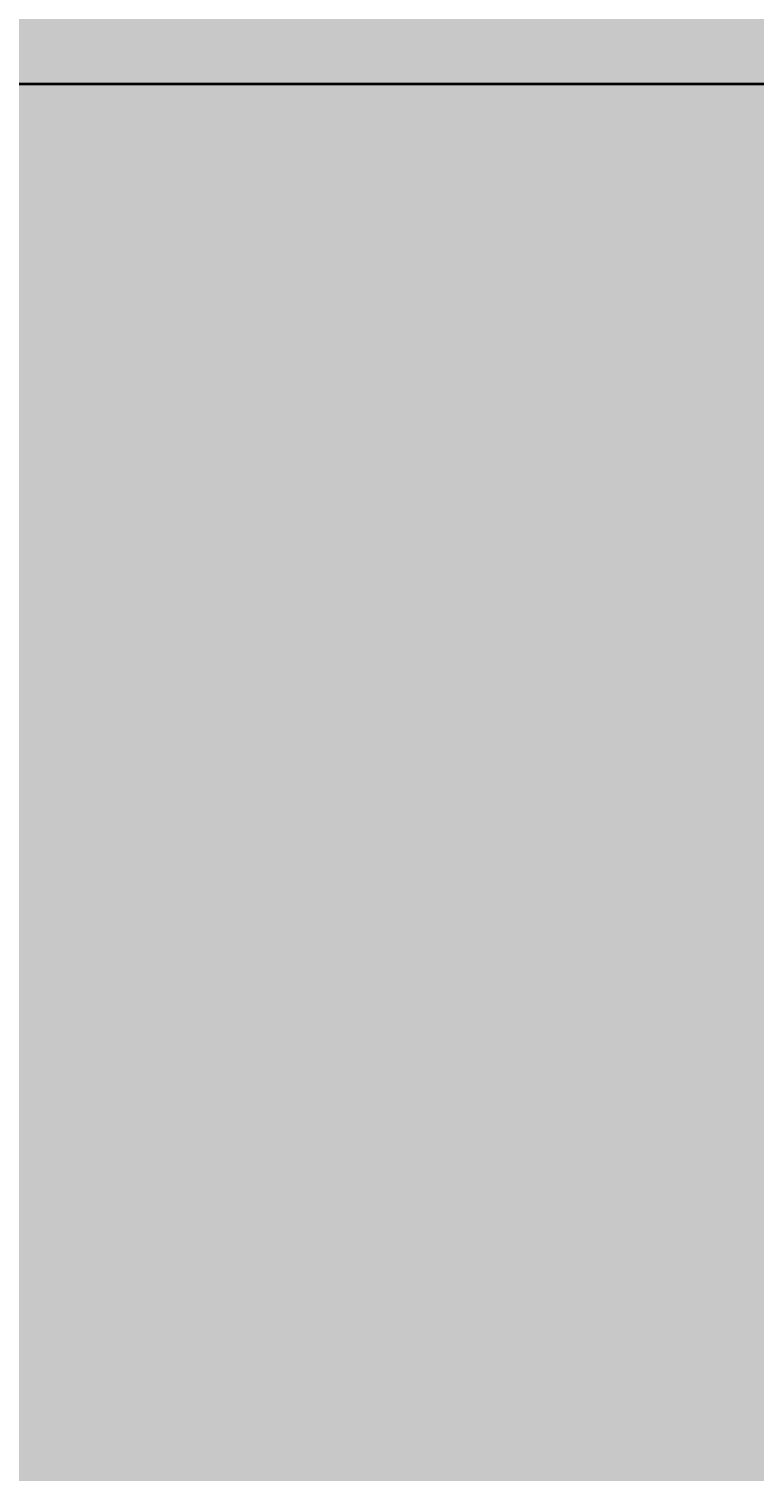
# Model space of a CAD drawing. Units: inches. Extents: x 84 to 1044, y -280 to 906.
# Tile 91 of 105: x 733 to 749, y 479 to 512. Entities that reach past the tile are written whole.
import ezdxf

# ---------------------------------------------------------------- set-up
doc = ezdxf.new("R2010")
doc.units = ezdxf.units.IN
doc.layers.add('A-ANNO-DIMS', color=2, linetype='Continuous', lineweight=18)
doc.layers.add('WALL', color=250, linetype='Continuous', lineweight=35)
doc.layers.add('A-WALL-PATT', color=251, linetype='Continuous', lineweight=9, true_color=0x636466)
doc.layers.add('L-PLNT-PATT', color=9, linetype='Continuous', lineweight=9, true_color=0xafd9aa)
doc.styles.get("Standard").update_dxf_attribs({"font": 'arial.ttf'})
doc.dimstyles.get("Standard").update_dxf_attribs({"dimtxt": 0.18, "dimasz": 0.18, "dimexe": 0.18, "dimexo": 0.0625, "dimgap": 0.09, "dimtad": 0, "dimtih": 1, "dimtoh": 1, "dimdec": 4, "dimzin": 0, "dimdsep": 46, "dimtxsty": 'Standard', "dimcen": 0.09, "dimadec": 0, "dimazin": 0, "dimtfac": 1, "dimtdec": 4, "dimtofl": 0, "dimtmove": 0, "dimatfit": 3, "dimfxl": 1, "dimtolj": 1, "dimtzin": 0, "dimarcsym": 0})

# ---------------------------------------------------------------- blocks, each defined once
blk = doc.blocks.new('*D62')
at = {"layer": 'A-ANNO-DIMS', "color": 0, "lineweight": -2, "transparency": 16777216}
for p, q in [((203.179, 709.183), (203.179, 905.9)), ((896.074, 400.183), (896.074, 905.9)), ((203.359, 905.72), (549.232, 905.72)), ((895.894, 905.72), (550.021, 905.72))]:
    blk.add_line(p, q, dxfattribs=at)
at = {"layer": 'A-ANNO-DIMS', "color": 0, "transparency": 16777216}
for points in [[(203.359, 905.75), (203.359, 905.69), (203.179, 905.72)], [(895.894, 905.75), (895.894, 905.69), (896.074, 905.72)]]:
    blk.add_solid(points, dxfattribs=at)
at = {"layer": 'Defpoints', "color": 0, "transparency": 16777216}
for p in [(896.074, 905.72), (203.179, 709.12), (896.074, 400.12)]:
    blk.add_point(p, dxfattribs=at)
at = {"layer": 'A-ANNO-DIMS', "color": 0, "transparency": 16777216, "insert": (549.627, 905.72), "char_height": 0.18, "attachment_point": 5}
blk.add_mtext('\\A1;692.9', dxfattribs=at)

msp = doc.modelspace()

# ---------------------------------------------------------------- hatches: boundary and pattern name
at = {"layer": 'A-WALL-PATT', "transparency": 33554597}
h = msp.add_hatch(color=256, dxfattribs=at)
h.dxf.hatch_style = 1
h.paths.add_polyline_path([(671.074, 100.12), (647.074, 100.12), (647.074, 160.12), (641.074, 160.12), (620.824, 160.12), (620.824, 151.12), (638.074, 151.12), (638.074, 91.12), (671.074, 91.12)])
h.paths.add_polyline_path([(791.074, 100.12), (743.074, 100.12), (743.074, 91.12), (791.074, 91.12)])
h.paths.add_polyline_path([(896.074, 346.12), (887.074, 346.12), (887.074, 334.12), (870.955, 334.12), (833.074, 334.12), (804.574, 334.12), (804.574, 328.12), (887.074, 328.12), (887.074, 100.12), (863.074, 100.12), (863.074, 91.12), (896.074, 91.12)])
h.paths.add_polyline_path([(507.574, 154.729), (507.574, 160.12), (464.074, 160.12), (464.074, 247.12), (641.074, 247.12), (641.074, 208.12), (647.074, 208.12), (647.074, 328.12), (659.074, 328.12), (659.074, 334.12), (617.074, 334.12), (617.074, 328.12), (641.074, 328.12), (641.074, 256.12), (545.074, 256.12), (545.074, 328.12), (569.074, 328.12), (569.074, 334.12), (518.074, 334.12), (518.074, 325.12), (536.074, 325.12), (536.074, 256.12), (464.074, 256.12), (464.074, 325.12), (482.074, 325.12), (482.074, 334.12), (455.074, 334.12), (455.074, 160.12), (413.127, 160.12), (413.127, 151.12), (455.074, 151.12), (455.074, 91.12), (464.074, 91.12), (464.074, 151.12), (507.574, 151.12)])
h.paths.add_polyline_path([(572.824, 160.12), (555.574, 160.12), (555.574, 151.12), (572.824, 151.12)], flags=17)
h.paths.add_polyline_path([(341.127, 160.12), (299.179, 160.12), (299.179, 211.12), (294.179, 211.12), (290.179, 211.12), (290.179, 151.12), (341.127, 151.12)])
h.paths.add_polyline_path([(299.179, 256.12), (212.179, 256.12), (212.179, 274.12), (203.179, 274.12), (203.179, 247.12), (299.179, 247.12)])
h.paths.add_polyline_path([(212.179, 514.12), (398.074, 514.12), (398.074, 519.12), (398.074, 520.12), (212.179, 520.12), (212.179, 574.12), (203.179, 574.12), (203.179, 310.12), (212.179, 310.12), (212.179, 328.12), (290.179, 328.12), (290.179, 292.12), (299.179, 292.12), (299.179, 328.12), (332.179, 328.12), (332.179, 334.12), (212.179, 334.12)])
h.paths.add_polyline_path([(287.127, 709.12), (203.179, 709.12), (203.179, 646.12), (212.179, 646.12), (212.179, 700.12), (287.127, 700.12)])
h.paths.add_polyline_path([(470.074, 709.12), (359.127, 709.12), (359.127, 700.12), (434.074, 700.12), (434.074, 574.12), (440.074, 574.12), (440.074, 622.12), (464.074, 622.12), (464.074, 628.12), (440.074, 628.12), (440.074, 700.12), (470.074, 700.12)])
h.paths.add_polyline_path([(572.074, 709.12), (506.074, 709.12), (506.074, 700.12), (536.074, 700.12), (536.074, 628.12), (494.074, 628.12), (494.074, 622.12), (536.074, 622.12), (536.074, 520.12), (440.074, 520.12), (440.074, 544.12), (434.074, 544.12), (434.074, 514.12), (644.074, 514.12), (644.074, 519.12), (644.074, 544.12), (638.074, 544.12), (638.074, 520.12), (542.074, 520.12), (542.074, 622.12), (584.074, 622.12), (584.074, 628.12), (542.074, 628.12), (542.074, 700.12), (572.074, 700.12)])
h.paths.add_polyline_path([(698.074, 709.12), (608.074, 709.12), (608.074, 700.12), (638.074, 700.12), (638.074, 628.12), (614.074, 628.12), (614.074, 622.12), (638.074, 622.12), (638.074, 574.12), (644.074, 574.12), (644.074, 700.12), (698.074, 700.12)])
h.paths.add_polyline_path([(833.074, 709.12), (770.074, 709.12), (770.074, 700.12), (824.074, 700.12), (824.074, 646.12), (833.074, 646.12)])
h.paths.add_polyline_path([(833.074, 574.12), (824.074, 574.12), (824.074, 520.12), (791.244, 520.12), (712.904, 520.12), (680.074, 520.12), (680.074, 514.12), (695.074, 514.12), (695.074, 491.62), (704.074, 491.62), (704.074, 511.12), (833.074, 511.12)])
h.paths.add_polyline_path([(704.074, 419.62), (695.074, 419.62), (695.074, 370.12), (704.074, 370.12)])
h.paths.add_polyline_path([(896.074, 400.12), (833.074, 400.12), (833.074, 364.12), (839.074, 364.12), (839.074, 394.12), (887.074, 394.12), (887.074, 382.12), (896.074, 382.12)])
h.paths.add_polyline_path([(732.574, 334.12), (695.074, 334.12), (695.074, 328.12), (732.574, 328.12)])
at = {"layer": 'L-PLNT-PATT', "transparency": 33554597}
h = msp.add_hatch(color=256, dxfattribs=at)
h.dxf.hatch_style = 1
h.paths.add_polyline_path([(896.074, 511.12), (704.074, 511.12), (704.074, 491.62), (704.074, 419.62), (704.074, 400.12), (833.074, 400.12), (896.074, 400.12)])

# ---------------------------------------------------------------- linework, layer by layer
at = {"layer": 'WALL'}
msp.add_line((896.074, 511.12), (704.074, 511.12), dxfattribs=at)

# ---------------------------------------------------------------- dimensions: what is measured, and where the dimension line sits
at = {"layer": 'A-ANNO-DIMS'}
dim = msp.add_linear_dim(base=(896.074, 905.72), p1=(203.179, 709.12), p2=(896.074, 400.12), dimstyle='Standard', override={"dimdec": 1, "dimlfac": 1, "dimrnd": 0, "dimzin": 0, "dimdsep": 46, "dimlunit": 2}, dxfattribs=at)
dim.commit()
dim.dimension.update_dxf_attribs({"geometry": '*D62', "text_midpoint": (549.627, 905.72)})

doc.saveas('drawing.dxf')
